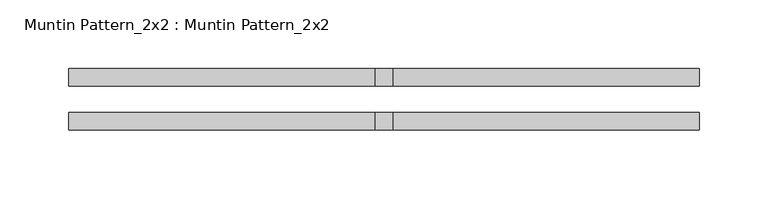
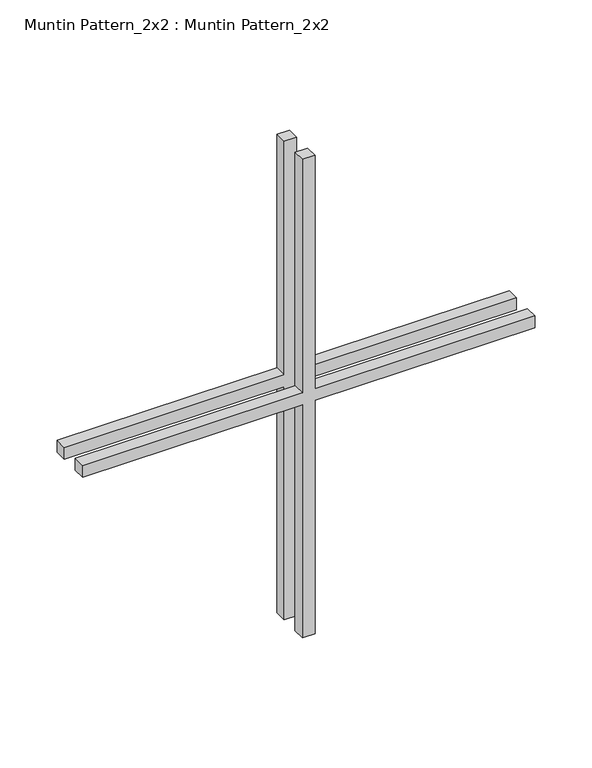
"""IFC4 building model written with IfcOpenShell, lengths in millimetres: proxy geometry, Muntin Pattern_2x2 : Muntin Pattern_2x2."""

from ifc_helpers import new_model, si_unit, frame, origin, place, context, project, spatial, polyline, outline, extrude, source, transform, mapped, element, save


def muntin_pattern_2x2_muntin_pattern_2x2_3440c8d2(model_context):
    return source(origin(), model_context, "Body", "SweptSolid", [
        extrude(outline(polyline([(261.9375, -6.35), (261.9375, -228.6), (249.2375, -228.6), (249.2375, -6.35), (0.0, -6.35), (0.0, 6.35), (249.2375, 6.35), (249.2375, 228.6), (261.9375, 228.6), (261.9375, 6.35), (511.175, 6.35), (511.175, -6.35), (261.9375, -6.35)])), frame((0.0, 9.525, 0.0), z_axis=(0.0, 1.0, 0.0), x_axis=(0.0, 0.0, 1.0)), (0.0, 0.0, 1.0), 12.7),
        extrude(outline(polyline([(261.9375, -6.35), (261.9375, -228.6), (249.2375, -228.6), (249.2375, -6.35), (0.0, -6.35), (0.0, 6.35), (249.2375, 6.35), (249.2375, 228.6), (261.9375, 228.6), (261.9375, 6.35), (511.175, 6.35), (511.175, -6.35), (261.9375, -6.35)])), frame((0.0, -22.225, 0.0), z_axis=(0.0, 1.0, 0.0), x_axis=(0.0, 0.0, 1.0)), (0.0, 0.0, 1.0), 12.7),
    ])


if __name__ == "__main__":
    model = new_model("IFC4")
    model_context = context("Model", 3, world=origin())
    ifc_project = project(units=[si_unit("LENGTHUNIT", "METRE", prefix="MILLI")], contexts=[model_context])
    site = spatial("IfcSite", under=ifc_project)
    building = spatial("IfcBuilding", under=site)
    placement = place(None, origin())
    muntin_pattern_2x2_muntin_pattern_2x2_shape = muntin_pattern_2x2_muntin_pattern_2x2_3440c8d2(model_context)
    element("IfcBuildingElementProxy", 1, Name="Muntin Pattern_2x2 : Muntin Pattern_2x2", ObjectType="Muntin Pattern_2x2 : Muntin Pattern_2x2", at=placement, inside=building, context=model_context, shape_type="MappedRepresentation", body=[
        mapped(muntin_pattern_2x2_muntin_pattern_2x2_shape, transform((0.0, 0.0, 0.0), x_axis=(1.0, 0.0, 0.0), y_axis=(0.0, 1.0, 0.0), z_axis=(0.0, 0.0, 1.0))),
    ])
    save(model, "model.ifc")

# Revit data of these elements
# Type "Muntin Pattern_2x2 : Muntin Pattern_2x2"
#   Width [instance default] = 4' - 0"
#   Thickness = 0' - 0 1/2"
#   Height [instance default] = 4' - 0"
#   Distance = 0' - 0 3/4"
#   Interior Material [instance default] = none
#   Exterior Material [instance default] = none
#   Default Elevation = 0
# Element 1 (IfcBuildingElementProxy, "Muntin Pattern_2x2 : Muntin Pattern_2x2")
#   Width = 1' - 6"
#   Height = 1' - 8 1/8"
#   Interior Material = Wood - Stained
#   Exterior Material = Clad - White
#   Materials on its faces: "Clad - White", "Wood - Stained"
# Materials
#   "Clad - White": class "Wood", colour RGB 242 242 238, transparency 0, Cost = 0
#   "Wood - Stained": class "Wood", colour RGB 224 178 126, transparency 0, Cost = 0
